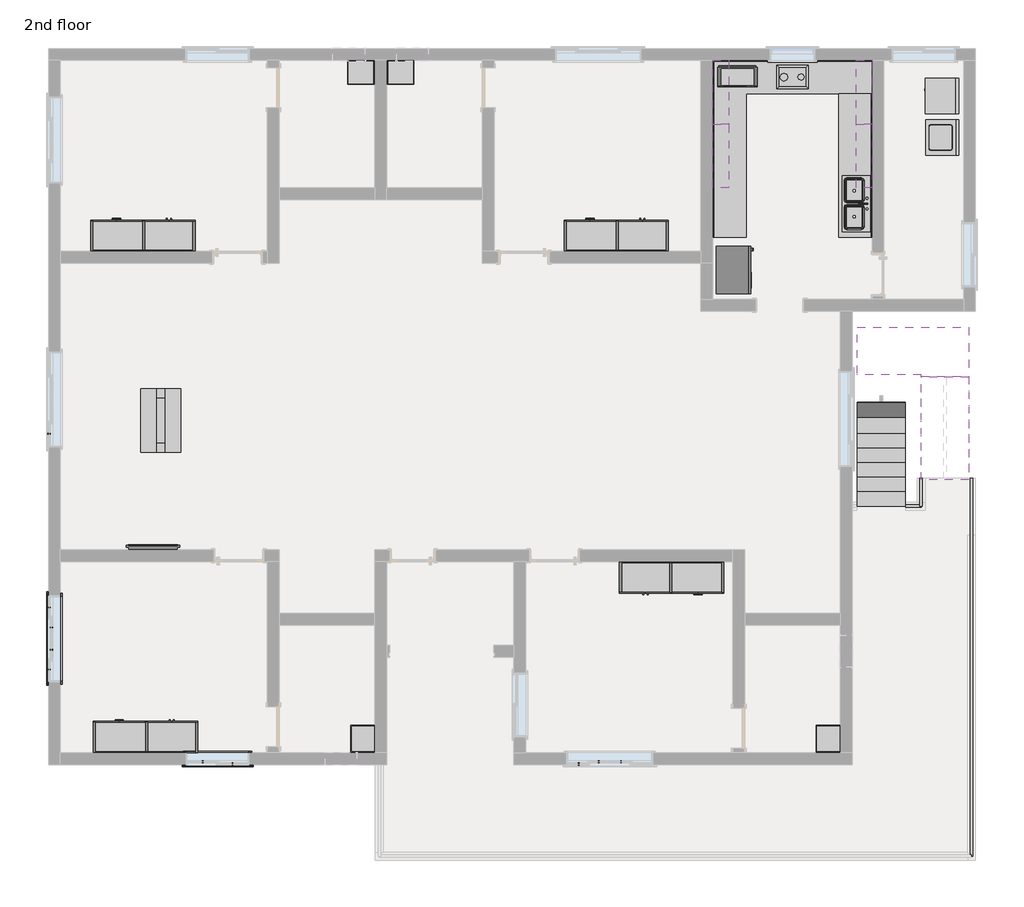
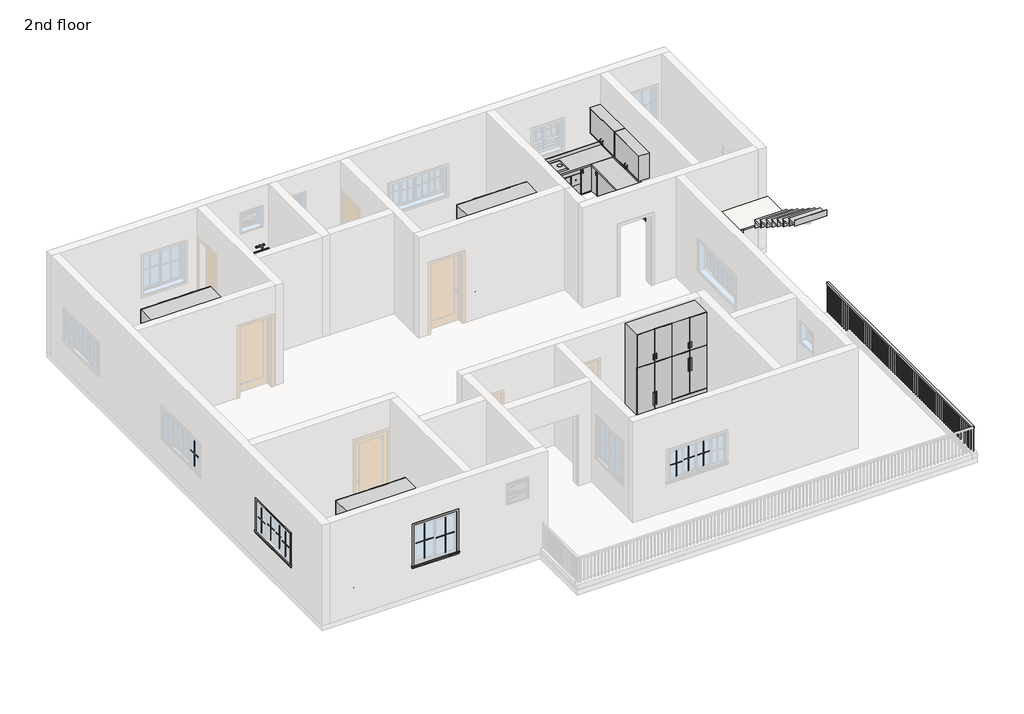
# One storey, part 3 of 4: 19 furniture elements, 18 proxies, 5 flow terminals, 3 railings, 2 stair flights, 1 slab.
"""IFC4 building model written with IfcOpenShell, lengths in millimetres."""

from ifc_helpers import new_model, si_unit, frame, origin, place, context, project, spatial, polyline, outline, extrude, transform, mapped, element, save
from components import proxy_3c1fa1d0, proxy_97c73763, proxy_e661f726, muntin_pattern_2x2_muntin_pattern_2x2_6186d23a, muntin_pattern_2x2_muntin_pattern_2x2_31a16349, muntin_pattern_2x2_muntin_pattern_2x2_cf37b409, trim_window_exterior_flat_with_sill_c3f87112, trim_window_exterior_flat_with_sill_7cfdd449, trim_window_interior_flat_picture_frame_1c33fa8a, trim_window_interior_flat_picture_frame_f1e0b15b, proxy_e75280ca, flow_terminal_cce4e9d2, flow_terminal_a53be723, furniture_65fa61b5, furniture_1wardrobe_6271_1wardrobe_6271_4dd35231, furniture_3428e43d, furniture_97fe820d, furniture_803bf5e8, furniture_2797bbf7, furniture_b6aab1a0, furniture_ea954fa4, white_modern_coffee_table_17067_white_modern_coffee_table_d4aed9ff, non_monolithic_landing_7206712e, stair_flight_52e4cb2b, stair_flight_4fb3dba1

model = new_model("IFC4")

# Units and contexts
model_context = context("Model", 3, world=origin())
ifc_project = project(units=[si_unit("LENGTHUNIT", "METRE", prefix="MILLI")], contexts=[model_context])

# Site, building, storey
site = spatial("IfcSite", under=ifc_project)
building = spatial("IfcBuilding", under=site)
storey = spatial("IfcBuildingStorey", under=building, Name="2nd floor", Elevation=7010.4)

# Proxies
placement = place(None, origin())
proxy_shape = proxy_3c1fa1d0(model_context)
element("IfcBuildingElementProxy", 1, Name="Cook Top-2 Unit : 12\" x 18\" 2", ObjectType="Cook Top-2 Unit : 12\" x 18\" 2", at=placement, inside=storey, context=model_context, shape_type="MappedRepresentation", body=[
    mapped(proxy_shape, transform((6250.0508793, 6451.6660813, 7010.4), x_axis=(0.0, 1.0, 0.0), y_axis=(-1.0, 0.0, 0.0), z_axis=(0.0, 0.0, 1.0))),
])
proxy_2_shape = proxy_97c73763(model_context)
element("IfcBuildingElementProxy", 2, Name="Dryer : 27\" x 25\" x 35\"", ObjectType="Dryer : 27\" x 25\" x 35\"", at=placement, inside=storey, context=model_context, shape_type="MappedRepresentation", body=[
    mapped(proxy_2_shape, transform((8769.6870876, 6542.578625, 7010.4), x_axis=(0.0, -1.0, 0.0), y_axis=(1.0, 0.0, 0.0), z_axis=(0.0, 0.0, 1.0))),
])
proxy_3_shape = proxy_e661f726(model_context)
element("IfcBuildingElementProxy", 3, Name="Microwave : 30\" x 16\" x 18\"", ObjectType="Microwave : 30\" x 16\" x 18\"", at=placement, inside=storey, context=model_context, shape_type="MappedRepresentation", body=[
    mapped(proxy_3_shape, transform((4665.4332064, 6893.6465872, 7010.4), x_axis=(1.0, 0.0, 0.0), y_axis=(0.0, 1.0, 0.0), z_axis=(0.0, 0.0, 1.0))),
])
muntin_pattern_2x2_muntin_pattern_2x2_shape = muntin_pattern_2x2_muntin_pattern_2x2_6186d23a(model_context)
element("IfcBuildingElementProxy", 4, Name="Muntin Pattern_2x2 : Muntin Pattern_2x2", ObjectType="Muntin Pattern_2x2 : Muntin Pattern_2x2", at=placement, inside=storey, context=model_context, shape_type="MappedRepresentation", body=[
    mapped(muntin_pattern_2x2_muntin_pattern_2x2_shape, transform((2933.7010838, -6588.0589187, 8007.35), x_axis=(-1.0, 0.0, 0.0), y_axis=(0.0, -1.0, 0.0), z_axis=(0.0, 0.0, 1.0))),
])
element("IfcBuildingElementProxy", 5, Name="Muntin Pattern_2x2 : Muntin Pattern_2x2", ObjectType="Muntin Pattern_2x2 : Muntin Pattern_2x2", at=placement, inside=storey, context=model_context, shape_type="MappedRepresentation", body=[
    mapped(muntin_pattern_2x2_muntin_pattern_2x2_shape, transform((2508.2510838, -6588.0589187, 8007.35), x_axis=(-1.0, 0.0, 0.0), y_axis=(0.0, -1.0, 0.0), z_axis=(0.0, 0.0, 1.0))),
])
element("IfcBuildingElementProxy", 6, Name="Muntin Pattern_2x2 : Muntin Pattern_2x2", ObjectType="Muntin Pattern_2x2 : Muntin Pattern_2x2", at=placement, inside=storey, context=model_context, shape_type="MappedRepresentation", body=[
    mapped(muntin_pattern_2x2_muntin_pattern_2x2_shape, transform((2127.2510838, -6632.5089187, 8007.35), x_axis=(-1.0, 0.0, 0.0), y_axis=(0.0, -1.0, 0.0), z_axis=(0.0, 0.0, 1.0))),
])
element("IfcBuildingElementProxy", 7, Name="Muntin Pattern_2x2 : Muntin Pattern_2x2", ObjectType="Muntin Pattern_2x2 : Muntin Pattern_2x2", at=placement, inside=storey, context=model_context, shape_type="MappedRepresentation", body=[
    mapped(muntin_pattern_2x2_muntin_pattern_2x2_shape, transform((-8020.0489162, -4822.7589187, 8007.35), x_axis=(0.0, 1.0, 0.0), y_axis=(-1.0, 0.0, 0.0), z_axis=(0.0, 0.0, 1.0))),
])
element("IfcBuildingElementProxy", 8, Name="Muntin Pattern_2x2 : Muntin Pattern_2x2", ObjectType="Muntin Pattern_2x2 : Muntin Pattern_2x2", at=placement, inside=storey, context=model_context, shape_type="MappedRepresentation", body=[
    mapped(muntin_pattern_2x2_muntin_pattern_2x2_shape, transform((-7975.5989162, -4441.7589187, 8007.35), x_axis=(0.0, 1.0, 0.0), y_axis=(-1.0, 0.0, 0.0), z_axis=(0.0, 0.0, 1.0))),
])
element("IfcBuildingElementProxy", 9, Name="Muntin Pattern_2x2 : Muntin Pattern_2x2", ObjectType="Muntin Pattern_2x2 : Muntin Pattern_2x2", at=placement, inside=storey, context=model_context, shape_type="MappedRepresentation", body=[
    mapped(muntin_pattern_2x2_muntin_pattern_2x2_shape, transform((-7975.5989162, -4016.3089187, 8007.35), x_axis=(0.0, 1.0, 0.0), y_axis=(-1.0, 0.0, 0.0), z_axis=(0.0, 0.0, 1.0))),
])
element("IfcBuildingElementProxy", 10, Name="Muntin Pattern_2x2 : Muntin Pattern_2x2", ObjectType="Muntin Pattern_2x2 : Muntin Pattern_2x2", at=placement, inside=storey, context=model_context, shape_type="MappedRepresentation", body=[
    mapped(muntin_pattern_2x2_muntin_pattern_2x2_shape, transform((-8020.0489162, -3635.3089187, 8007.35), x_axis=(0.0, 1.0, 0.0), y_axis=(-1.0, 0.0, 0.0), z_axis=(0.0, 0.0, 1.0))),
])
muntin_pattern_2x2_muntin_pattern_2x2_2_shape = muntin_pattern_2x2_muntin_pattern_2x2_31a16349(model_context)
element("IfcBuildingElementProxy", 11, Name="Muntin Pattern_2x2 : Muntin Pattern_2x2", ObjectType="Muntin Pattern_2x2 : Muntin Pattern_2x2", at=placement, inside=storey, context=model_context, shape_type="MappedRepresentation", body=[
    mapped(muntin_pattern_2x2_muntin_pattern_2x2_2_shape, transform((-8020.0489162, -304.7339187, 8007.35), x_axis=(0.0, 1.0, 0.0), y_axis=(-1.0, 0.0, 0.0), z_axis=(0.0, 0.0, 1.0))),
])
muntin_pattern_2x2_muntin_pattern_2x2_3_shape = muntin_pattern_2x2_muntin_pattern_2x2_cf37b409(model_context)
element("IfcBuildingElementProxy", 12, Name="Muntin Pattern_2x2 : Muntin Pattern_2x2", ObjectType="Muntin Pattern_2x2 : Muntin Pattern_2x2", at=placement, inside=storey, context=model_context, shape_type="MappedRepresentation", body=[
    mapped(muntin_pattern_2x2_muntin_pattern_2x2_3_shape, transform((-5075.2364162, -6588.0589187, 8007.35), x_axis=(-1.0, 0.0, 0.0), y_axis=(0.0, -1.0, 0.0), z_axis=(0.0, 0.0, 1.0))),
])
element("IfcBuildingElementProxy", 13, Name="Muntin Pattern_2x2 : Muntin Pattern_2x2", ObjectType="Muntin Pattern_2x2 : Muntin Pattern_2x2", at=placement, inside=storey, context=model_context, shape_type="MappedRepresentation", body=[
    mapped(muntin_pattern_2x2_muntin_pattern_2x2_3_shape, transform((-4506.9114162, -6632.5089187, 8007.35), x_axis=(-1.0, 0.0, 0.0), y_axis=(0.0, -1.0, 0.0), z_axis=(0.0, 0.0, 1.0))),
])
trim_window_exterior_flat_with_sill_shape = trim_window_exterior_flat_with_sill_c3f87112(model_context)
element("IfcBuildingElementProxy", 14, Name="Trim-Window-Exterior-Flat : with Sill", ObjectType="Trim-Window-Exterior-Flat : with Sill", at=placement, inside=storey, context=model_context, shape_type="MappedRepresentation", body=[
    mapped(trim_window_exterior_flat_with_sill_shape, transform((-8029.5739162, -4229.0339187, 8839.2), x_axis=(0.0, -1.0, 0.0), y_axis=(0.0, 0.0, 1.0), z_axis=(-1.0, 0.0, 0.0))),
])
trim_window_exterior_flat_with_sill_2_shape = trim_window_exterior_flat_with_sill_7cfdd449(model_context)
element("IfcBuildingElementProxy", 15, Name="Trim-Window-Exterior-Flat : with Sill", ObjectType="Trim-Window-Exterior-Flat : with Sill", at=placement, inside=storey, context=model_context, shape_type="MappedRepresentation", body=[
    mapped(trim_window_exterior_flat_with_sill_2_shape, transform((-4791.0739162, -6642.0339187, 9144.0), x_axis=(1.0, 0.0, 0.0), y_axis=(0.0, 0.0, 1.0), z_axis=(0.0, -1.0, 0.0))),
])
trim_window_interior_flat_picture_frame_shape = trim_window_interior_flat_picture_frame_1c33fa8a(model_context)
element("IfcBuildingElementProxy", 16, Name="Trim-Window-Interior-Flat : Picture Frame", ObjectType="Trim-Window-Interior-Flat : Picture Frame", at=placement, inside=storey, context=model_context, shape_type="MappedRepresentation", body=[
    mapped(trim_window_interior_flat_picture_frame_shape, transform((-7800.9739162, -4229.0339187, 8839.2), x_axis=(0.0, 1.0, 0.0), y_axis=(0.0, 0.0, 1.0), z_axis=(1.0, 0.0, 0.0))),
])
trim_window_interior_flat_picture_frame_2_shape = trim_window_interior_flat_picture_frame_f1e0b15b(model_context)
element("IfcBuildingElementProxy", 17, Name="Trim-Window-Interior-Flat : Picture Frame", ObjectType="Trim-Window-Interior-Flat : Picture Frame", at=placement, inside=storey, context=model_context, shape_type="MappedRepresentation", body=[
    mapped(trim_window_interior_flat_picture_frame_2_shape, transform((-4791.0739162, -6413.4339187, 9144.0), x_axis=(-1.0, 0.0, 0.0), y_axis=(0.0, 0.0, 1.0), z_axis=(0.0, 1.0, 0.0))),
])
proxy_4_shape = proxy_e75280ca(model_context)
element("IfcBuildingElementProxy", 18, Name="Washer : 27\" x 25\" x 35\"", ObjectType="Washer : 27\" x 25\" x 35\"", at=placement, inside=storey, context=model_context, shape_type="MappedRepresentation", body=[
    mapped(proxy_4_shape, transform((8810.3756486, 5789.9486128, 7010.4), x_axis=(0.0, -1.0, 0.0), y_axis=(1.0, 0.0, 0.0), z_axis=(0.0, 0.0, 1.0))),
])

# Flow terminals
flow_terminal_shape = flow_terminal_cce4e9d2(model_context)
element("IfcFlowTerminal", 19, ObjectType="Sink - Work : 20\"x18\"", at=placement, inside=storey, context=model_context, shape_type="MappedRepresentation", body=[
    mapped(flow_terminal_shape, transform((-1285.8739162, 6845.3660813, 7924.8), x_axis=(1.0, 0.0, 0.0), y_axis=(0.0, 1.0, 0.0), z_axis=(0.0, 0.0, 1.0))),
])
element("IfcFlowTerminal", 20, ObjectType="Sink - Work : 20\"x18\"", at=placement, inside=storey, context=model_context, shape_type="MappedRepresentation", body=[
    mapped(flow_terminal_shape, transform((-2047.8739162, 6845.3660813, 7924.8), x_axis=(1.0, 0.0, 0.0), y_axis=(0.0, 1.0, 0.0), z_axis=(0.0, 0.0, 1.0))),
])
element("IfcFlowTerminal", 21, ObjectType="Sink - Work : 20\"x18\"", at=placement, inside=storey, context=model_context, shape_type="MappedRepresentation", body=[
    mapped(flow_terminal_shape, transform((-1781.1739162, -6146.7339187, 7924.8), x_axis=(0.0, -1.0, 0.0), y_axis=(1.0, 0.0, 0.0), z_axis=(0.0, 0.0, 1.0))),
])
element("IfcFlowTerminal", 22, ObjectType="Sink - Work : 20\"x18\"", at=placement, inside=storey, context=model_context, shape_type="MappedRepresentation", body=[
    mapped(flow_terminal_shape, transform((7134.2260838, -6146.7339187, 7924.8), x_axis=(0.0, -1.0, 0.0), y_axis=(1.0, 0.0, 0.0), z_axis=(0.0, 0.0, 1.0))),
])
flow_terminal_2_shape = flow_terminal_a53be723(model_context)
element("IfcFlowTerminal", 23, ObjectType="Sink Kitchen-Double : 42\" x 21\"", at=placement, inside=storey, context=model_context, shape_type="MappedRepresentation", body=[
    mapped(flow_terminal_2_shape, transform((7436.6806826, 4117.8553219, 7010.4), x_axis=(0.0, -1.0, 0.0), y_axis=(1.0, 0.0, 0.0), z_axis=(0.0, 0.0, 1.0))),
])

# Furniture
furniture_shape = furniture_65fa61b5(model_context)
element("IfcFurniture", 24, at=placement, inside=storey, context=model_context, shape_type="MappedRepresentation", body=[
    mapped(furniture_shape, transform((4759.3260838, 3441.7660813, 7010.4), x_axis=(0.0, 1.0, 0.0), y_axis=(-1.0, 0.0, 0.0), z_axis=(0.0, 0.0, 1.0))),
])
furniture_1wardrobe_6271_1wardrobe_6271_shape = furniture_1wardrobe_6271_1wardrobe_6271_4dd35231(model_context)
element("IfcFurniture", 25, ObjectType="1Wardrobe_6271 : 1Wardrobe_6271", at=placement, inside=storey, context=model_context, shape_type="MappedRepresentation", body=[
    mapped(furniture_1wardrobe_6271_1wardrobe_6271_shape, transform((-5222.8739162, 3187.7660813, 7010.4), x_axis=(-1.0, 0.0, 0.0), y_axis=(0.0, -1.0, 0.0), z_axis=(0.0, 0.0, 1.0))),
])
element("IfcFurniture", 26, ObjectType="1Wardrobe_6271 : 1Wardrobe_6271", at=placement, inside=storey, context=model_context, shape_type="MappedRepresentation", body=[
    mapped(furniture_1wardrobe_6271_1wardrobe_6271_shape, transform((3844.9260838, 3187.7660813, 7010.4), x_axis=(-1.0, 0.0, 0.0), y_axis=(0.0, -1.0, 0.0), z_axis=(0.0, 0.0, 1.0))),
])
element("IfcFurniture", 27, ObjectType="1Wardrobe_6271 : 1Wardrobe_6271", at=placement, inside=storey, context=model_context, shape_type="MappedRepresentation", body=[
    mapped(furniture_1wardrobe_6271_1wardrobe_6271_shape, transform((2905.1260838, -2755.8339187, 7010.4), x_axis=(1.0, 0.0, 0.0), y_axis=(0.0, 1.0, 0.0), z_axis=(0.0, 0.0, 1.0))),
])
element("IfcFurniture", 28, ObjectType="1Wardrobe_6271 : 1Wardrobe_6271", at=placement, inside=storey, context=model_context, shape_type="MappedRepresentation", body=[
    mapped(furniture_1wardrobe_6271_1wardrobe_6271_shape, transform((-5172.0739162, -6413.4339187, 7010.4), x_axis=(-1.0, 0.0, 0.0), y_axis=(0.0, -1.0, 0.0), z_axis=(0.0, 0.0, 1.0))),
])
furniture_2_shape = furniture_3428e43d(model_context)
element("IfcFurniture", 29, ObjectType="48\" 2", at=placement, inside=storey, context=model_context, shape_type="MappedRepresentation", body=[
    mapped(furniture_2_shape, transform((6128.9811238, 6845.3660813, 7010.4), x_axis=(1.0, 0.0, 0.0), y_axis=(0.0, 1.0, 0.0), z_axis=(0.0, 0.0, 1.0))),
])
element("IfcFurniture", 30, ObjectType="48\" 2", at=placement, inside=storey, context=model_context, shape_type="MappedRepresentation", body=[
    mapped(furniture_2_shape, transform((7134.2260838, 5230.5211213, 7010.4), x_axis=(0.0, 1.0, 0.0), y_axis=(-1.0, 0.0, 0.0), z_axis=(0.0, 0.0, 1.0))),
])
element("IfcFurniture", 31, ObjectType="48\" 2", at=placement, inside=storey, context=model_context, shape_type="MappedRepresentation", body=[
    mapped(furniture_2_shape, transform((4695.8260838, 5230.5211213, 7010.4), x_axis=(0.0, 1.0, 0.0), y_axis=(-1.0, 0.0, 0.0), z_axis=(0.0, 0.0, 1.0))),
])
element("IfcFurniture", 32, ObjectType="48\" 2", at=placement, inside=storey, context=model_context, shape_type="MappedRepresentation", body=[
    mapped(furniture_2_shape, transform((4695.8260838, 4011.3211213, 7010.4), x_axis=(0.0, 1.0, 0.0), y_axis=(-1.0, 0.0, 0.0), z_axis=(0.0, 0.0, 1.0))),
])
furniture_3_shape = furniture_97fe820d(model_context)
element("IfcFurniture", 33, ObjectType="Base Cabinet-Corner Unit-Square : 36\"", at=placement, inside=storey, context=model_context, shape_type="MappedRepresentation", body=[
    mapped(furniture_3_shape, transform((7217.0883788, 6845.3660813, 7010.4), x_axis=(1.0, 0.0, 0.0), y_axis=(0.0, 1.0, 0.0), z_axis=(0.0, 0.0, 1.0))),
])
element("IfcFurniture", 34, ObjectType="Base Cabinet-Corner Unit-Square : 36\"", at=placement, inside=storey, context=model_context, shape_type="MappedRepresentation", body=[
    mapped(furniture_3_shape, transform((4695.8260838, 6318.6283764, 7010.4), x_axis=(0.0, 1.0, 0.0), y_axis=(-1.0, 0.0, 0.0), z_axis=(0.0, 0.0, 1.0))),
])
furniture_4_shape = furniture_803bf5e8(model_context)
element("IfcFurniture", 35, ObjectType="Counter Top w Sink : 24\" Depth", at=placement, inside=storey, context=model_context, shape_type="MappedRepresentation", body=[
    mapped(furniture_4_shape, transform((7743.8260838, 5009.9037862, 7010.4), x_axis=(0.0, -1.0, 0.0), y_axis=(1.0, 0.0, 0.0), z_axis=(0.0, 0.0, 1.0))),
])
furniture_5_shape = furniture_2797bbf7(model_context)
element("IfcFurniture", 36, ObjectType="Counter Top-L Shaped : 24\" Depth", at=placement, inside=storey, context=model_context, shape_type="MappedRepresentation", body=[
    mapped(furniture_5_shape, transform((5896.2883788, 6845.3660813, 7010.4), x_axis=(1.0, 0.0, 0.0), y_axis=(0.0, 1.0, 0.0), z_axis=(0.0, 0.0, 1.0))),
])
furniture_6_shape = furniture_b6aab1a0(model_context)
element("IfcFurniture", 37, ObjectType="Television-Plasma : 42\"", at=placement, inside=storey, context=model_context, shape_type="MappedRepresentation", body=[
    mapped(furniture_6_shape, transform((-5972.1739162, -2527.2339187, 8077.2), x_axis=(-1.0, 0.0, 0.0), y_axis=(0.0, -1.0, 0.0), z_axis=(0.0, 0.0, 1.0))),
])
furniture_7_shape = furniture_ea954fa4(model_context)
element("IfcFurniture", 38, ObjectType="Upper Cabinet-Pass-Thru : 48\" x 30\" x 12\"", at=placement, inside=storey, context=model_context, shape_type="MappedRepresentation", body=[
    mapped(furniture_7_shape, transform((4695.8260838, 6217.0283764, 7010.4), x_axis=(0.0, 1.0, 0.0), y_axis=(-1.0, 0.0, 0.0), z_axis=(0.0, 0.0, 1.0))),
])
element("IfcFurniture", 39, ObjectType="Upper Cabinet-Pass-Thru : 48\" x 30\" x 12\"", at=placement, inside=storey, context=model_context, shape_type="MappedRepresentation", body=[
    mapped(furniture_7_shape, transform((4695.8260838, 4997.8283764, 7010.4), x_axis=(0.0, 1.0, 0.0), y_axis=(-1.0, 0.0, 0.0), z_axis=(0.0, 0.0, 1.0))),
])
element("IfcFurniture", 40, ObjectType="Upper Cabinet-Pass-Thru : 48\" x 30\" x 12\"", at=placement, inside=storey, context=model_context, shape_type="MappedRepresentation", body=[
    mapped(furniture_7_shape, transform((7743.8260838, 6254.5037862, 7010.4), x_axis=(0.0, -1.0, 0.0), y_axis=(1.0, 0.0, 0.0), z_axis=(0.0, 0.0, 1.0))),
])
element("IfcFurniture", 41, ObjectType="Upper Cabinet-Pass-Thru : 48\" x 30\" x 12\"", at=placement, inside=storey, context=model_context, shape_type="MappedRepresentation", body=[
    mapped(furniture_7_shape, transform((7743.8260838, 5035.3037862, 7010.4), x_axis=(0.0, -1.0, 0.0), y_axis=(1.0, 0.0, 0.0), z_axis=(0.0, 0.0, 1.0))),
])
white_modern_coffee_table_17067_white_modern_coffee_table_shape = white_modern_coffee_table_17067_white_modern_coffee_table_d4aed9ff(model_context)
element("IfcFurniture", 42, ObjectType="White_Modern_Coffee_Table_17067 : White_Modern_Coffee_Table_17067", at=placement, inside=storey, context=model_context, shape_type="MappedRepresentation", body=[
    mapped(white_modern_coffee_table_17067_white_modern_coffee_table_shape, transform((-5878.4127262, -50.7339187, 7010.4), x_axis=(0.0, 1.0, 0.0), y_axis=(-1.0, 0.0, 0.0), z_axis=(0.0, 0.0, 1.0))),
])

# Railings
element("IfcRailing", 43, ObjectType="Handrail - Rectangular", at=placement, inside=storey, context=model_context, shape_type="SweptSolid", body=[
    extrude(outline(polyline([(9623.4260838, -1155.6339187), (9674.2260838, -1155.6339187), (9674.2260838, -8394.6339187), (9623.4260838, -8394.6339187), (9623.4260838, -1155.6339187)])), frame((0.0, 0.0, 7874.0), z_axis=(0.0, 0.0, 1.0), x_axis=(1.0, 0.0, 0.0)), (0.0, 0.0, 1.0), 50.8),
    extrude(outline(polyline([(9639.3010838, -8359.7089187), (9658.3510838, -8359.7089187), (9658.3510838, -8378.7589187), (9639.3010838, -8378.7589187), (9639.3010838, -8359.7089187)])), frame((0.0, 0.0, 7010.4), z_axis=(0.0, 0.0, 1.0), x_axis=(1.0, 0.0, 0.0)), (0.0, 0.0, 1.0), 863.6),
    extrude(outline(polyline([(9639.3010838, -8258.1089187), (9658.3510838, -8258.1089187), (9658.3510838, -8277.1589187), (9639.3010838, -8277.1589187), (9639.3010838, -8258.1089187)])), frame((0.0, 0.0, 7010.4), z_axis=(0.0, 0.0, 1.0), x_axis=(1.0, 0.0, 0.0)), (0.0, 0.0, 1.0), 863.6),
    extrude(outline(polyline([(9639.3010838, -8156.5089187), (9658.3510838, -8156.5089187), (9658.3510838, -8175.5589187), (9639.3010838, -8175.5589187), (9639.3010838, -8156.5089187)])), frame((0.0, 0.0, 7010.4), z_axis=(0.0, 0.0, 1.0), x_axis=(1.0, 0.0, 0.0)), (0.0, 0.0, 1.0), 863.6),
    extrude(outline(polyline([(9639.3010838, -8054.9089187), (9658.3510838, -8054.9089187), (9658.3510838, -8073.9589187), (9639.3010838, -8073.9589187), (9639.3010838, -8054.9089187)])), frame((0.0, 0.0, 7010.4), z_axis=(0.0, 0.0, 1.0), x_axis=(1.0, 0.0, 0.0)), (0.0, 0.0, 1.0), 863.6),
    extrude(outline(polyline([(9639.3010838, -7953.3089187), (9658.3510838, -7953.3089187), (9658.3510838, -7972.3589187), (9639.3010838, -7972.3589187), (9639.3010838, -7953.3089187)])), frame((0.0, 0.0, 7010.4), z_axis=(0.0, 0.0, 1.0), x_axis=(1.0, 0.0, 0.0)), (0.0, 0.0, 1.0), 863.6),
    extrude(outline(polyline([(9639.3010838, -7851.7089187), (9658.3510838, -7851.7089187), (9658.3510838, -7870.7589187), (9639.3010838, -7870.7589187), (9639.3010838, -7851.7089187)])), frame((0.0, 0.0, 7010.4), z_axis=(0.0, 0.0, 1.0), x_axis=(1.0, 0.0, 0.0)), (0.0, 0.0, 1.0), 863.6),
    extrude(outline(polyline([(9639.3010838, -7750.1089187), (9658.3510838, -7750.1089187), (9658.3510838, -7769.1589187), (9639.3010838, -7769.1589187), (9639.3010838, -7750.1089187)])), frame((0.0, 0.0, 7010.4), z_axis=(0.0, 0.0, 1.0), x_axis=(1.0, 0.0, 0.0)), (0.0, 0.0, 1.0), 863.6),
    extrude(outline(polyline([(9639.3010838, -7648.5089187), (9658.3510838, -7648.5089187), (9658.3510838, -7667.5589187), (9639.3010838, -7667.5589187), (9639.3010838, -7648.5089187)])), frame((0.0, 0.0, 7010.4), z_axis=(0.0, 0.0, 1.0), x_axis=(1.0, 0.0, 0.0)), (0.0, 0.0, 1.0), 863.6),
    extrude(outline(polyline([(9639.3010838, -7546.9089187), (9658.3510838, -7546.9089187), (9658.3510838, -7565.9589187), (9639.3010838, -7565.9589187), (9639.3010838, -7546.9089187)])), frame((0.0, 0.0, 7010.4), z_axis=(0.0, 0.0, 1.0), x_axis=(1.0, 0.0, 0.0)), (0.0, 0.0, 1.0), 863.6),
    extrude(outline(polyline([(9639.3010838, -7445.3089187), (9658.3510838, -7445.3089187), (9658.3510838, -7464.3589187), (9639.3010838, -7464.3589187), (9639.3010838, -7445.3089187)])), frame((0.0, 0.0, 7010.4), z_axis=(0.0, 0.0, 1.0), x_axis=(1.0, 0.0, 0.0)), (0.0, 0.0, 1.0), 863.6),
    extrude(outline(polyline([(9639.3010838, -7343.7089187), (9658.3510838, -7343.7089187), (9658.3510838, -7362.7589187), (9639.3010838, -7362.7589187), (9639.3010838, -7343.7089187)])), frame((0.0, 0.0, 7010.4), z_axis=(0.0, 0.0, 1.0), x_axis=(1.0, 0.0, 0.0)), (0.0, 0.0, 1.0), 863.6),
    extrude(outline(polyline([(9639.3010838, -7242.1089187), (9658.3510838, -7242.1089187), (9658.3510838, -7261.1589187), (9639.3010838, -7261.1589187), (9639.3010838, -7242.1089187)])), frame((0.0, 0.0, 7010.4), z_axis=(0.0, 0.0, 1.0), x_axis=(1.0, 0.0, 0.0)), (0.0, 0.0, 1.0), 863.6),
    extrude(outline(polyline([(9639.3010838, -7140.5089187), (9658.3510838, -7140.5089187), (9658.3510838, -7159.5589187), (9639.3010838, -7159.5589187), (9639.3010838, -7140.5089187)])), frame((0.0, 0.0, 7010.4), z_axis=(0.0, 0.0, 1.0), x_axis=(1.0, 0.0, 0.0)), (0.0, 0.0, 1.0), 863.6),
    extrude(outline(polyline([(9639.3010838, -7038.9089187), (9658.3510838, -7038.9089187), (9658.3510838, -7057.9589187), (9639.3010838, -7057.9589187), (9639.3010838, -7038.9089187)])), frame((0.0, 0.0, 7010.4), z_axis=(0.0, 0.0, 1.0), x_axis=(1.0, 0.0, 0.0)), (0.0, 0.0, 1.0), 863.6),
    extrude(outline(polyline([(9639.3010838, -6937.3089187), (9658.3510838, -6937.3089187), (9658.3510838, -6956.3589187), (9639.3010838, -6956.3589187), (9639.3010838, -6937.3089187)])), frame((0.0, 0.0, 7010.4), z_axis=(0.0, 0.0, 1.0), x_axis=(1.0, 0.0, 0.0)), (0.0, 0.0, 1.0), 863.6),
    extrude(outline(polyline([(9639.3010838, -6835.7089187), (9658.3510838, -6835.7089187), (9658.3510838, -6854.7589187), (9639.3010838, -6854.7589187), (9639.3010838, -6835.7089187)])), frame((0.0, 0.0, 7010.4), z_axis=(0.0, 0.0, 1.0), x_axis=(1.0, 0.0, 0.0)), (0.0, 0.0, 1.0), 863.6),
    extrude(outline(polyline([(9639.3010838, -6734.1089187), (9658.3510838, -6734.1089187), (9658.3510838, -6753.1589187), (9639.3010838, -6753.1589187), (9639.3010838, -6734.1089187)])), frame((0.0, 0.0, 7010.4), z_axis=(0.0, 0.0, 1.0), x_axis=(1.0, 0.0, 0.0)), (0.0, 0.0, 1.0), 863.6),
    extrude(outline(polyline([(9639.3010838, -6632.5089187), (9658.3510838, -6632.5089187), (9658.3510838, -6651.5589187), (9639.3010838, -6651.5589187), (9639.3010838, -6632.5089187)])), frame((0.0, 0.0, 7010.4), z_axis=(0.0, 0.0, 1.0), x_axis=(1.0, 0.0, 0.0)), (0.0, 0.0, 1.0), 863.6),
    extrude(outline(polyline([(9639.3010838, -6530.9089187), (9658.3510838, -6530.9089187), (9658.3510838, -6549.9589187), (9639.3010838, -6549.9589187), (9639.3010838, -6530.9089187)])), frame((0.0, 0.0, 7010.4), z_axis=(0.0, 0.0, 1.0), x_axis=(1.0, 0.0, 0.0)), (0.0, 0.0, 1.0), 863.6),
    extrude(outline(polyline([(9639.3010838, -6429.3089187), (9658.3510838, -6429.3089187), (9658.3510838, -6448.3589187), (9639.3010838, -6448.3589187), (9639.3010838, -6429.3089187)])), frame((0.0, 0.0, 7010.4), z_axis=(0.0, 0.0, 1.0), x_axis=(1.0, 0.0, 0.0)), (0.0, 0.0, 1.0), 863.6),
    extrude(outline(polyline([(9639.3010838, -6327.7089187), (9658.3510838, -6327.7089187), (9658.3510838, -6346.7589187), (9639.3010838, -6346.7589187), (9639.3010838, -6327.7089187)])), frame((0.0, 0.0, 7010.4), z_axis=(0.0, 0.0, 1.0), x_axis=(1.0, 0.0, 0.0)), (0.0, 0.0, 1.0), 863.6),
    extrude(outline(polyline([(9639.3010838, -6226.1089187), (9658.3510838, -6226.1089187), (9658.3510838, -6245.1589187), (9639.3010838, -6245.1589187), (9639.3010838, -6226.1089187)])), frame((0.0, 0.0, 7010.4), z_axis=(0.0, 0.0, 1.0), x_axis=(1.0, 0.0, 0.0)), (0.0, 0.0, 1.0), 863.6),
    extrude(outline(polyline([(9639.3010838, -6124.5089187), (9658.3510838, -6124.5089187), (9658.3510838, -6143.5589187), (9639.3010838, -6143.5589187), (9639.3010838, -6124.5089187)])), frame((0.0, 0.0, 7010.4), z_axis=(0.0, 0.0, 1.0), x_axis=(1.0, 0.0, 0.0)), (0.0, 0.0, 1.0), 863.6),
    extrude(outline(polyline([(9639.3010838, -6022.9089187), (9658.3510838, -6022.9089187), (9658.3510838, -6041.9589187), (9639.3010838, -6041.9589187), (9639.3010838, -6022.9089187)])), frame((0.0, 0.0, 7010.4), z_axis=(0.0, 0.0, 1.0), x_axis=(1.0, 0.0, 0.0)), (0.0, 0.0, 1.0), 863.6),
    extrude(outline(polyline([(9639.3010838, -5921.3089187), (9658.3510838, -5921.3089187), (9658.3510838, -5940.3589187), (9639.3010838, -5940.3589187), (9639.3010838, -5921.3089187)])), frame((0.0, 0.0, 7010.4), z_axis=(0.0, 0.0, 1.0), x_axis=(1.0, 0.0, 0.0)), (0.0, 0.0, 1.0), 863.6),
    extrude(outline(polyline([(9639.3010838, -5819.7089187), (9658.3510838, -5819.7089187), (9658.3510838, -5838.7589187), (9639.3010838, -5838.7589187), (9639.3010838, -5819.7089187)])), frame((0.0, 0.0, 7010.4), z_axis=(0.0, 0.0, 1.0), x_axis=(1.0, 0.0, 0.0)), (0.0, 0.0, 1.0), 863.6),
    extrude(outline(polyline([(9639.3010838, -5718.1089187), (9658.3510838, -5718.1089187), (9658.3510838, -5737.1589187), (9639.3010838, -5737.1589187), (9639.3010838, -5718.1089187)])), frame((0.0, 0.0, 7010.4), z_axis=(0.0, 0.0, 1.0), x_axis=(1.0, 0.0, 0.0)), (0.0, 0.0, 1.0), 863.6),
    extrude(outline(polyline([(9639.3010838, -5616.5089187), (9658.3510838, -5616.5089187), (9658.3510838, -5635.5589187), (9639.3010838, -5635.5589187), (9639.3010838, -5616.5089187)])), frame((0.0, 0.0, 7010.4), z_axis=(0.0, 0.0, 1.0), x_axis=(1.0, 0.0, 0.0)), (0.0, 0.0, 1.0), 863.6),
    extrude(outline(polyline([(9639.3010838, -5514.9089187), (9658.3510838, -5514.9089187), (9658.3510838, -5533.9589187), (9639.3010838, -5533.9589187), (9639.3010838, -5514.9089187)])), frame((0.0, 0.0, 7010.4), z_axis=(0.0, 0.0, 1.0), x_axis=(1.0, 0.0, 0.0)), (0.0, 0.0, 1.0), 863.6),
    extrude(outline(polyline([(9639.3010838, -5413.3089187), (9658.3510838, -5413.3089187), (9658.3510838, -5432.3589187), (9639.3010838, -5432.3589187), (9639.3010838, -5413.3089187)])), frame((0.0, 0.0, 7010.4), z_axis=(0.0, 0.0, 1.0), x_axis=(1.0, 0.0, 0.0)), (0.0, 0.0, 1.0), 863.6),
    extrude(outline(polyline([(9639.3010838, -5311.7089187), (9658.3510838, -5311.7089187), (9658.3510838, -5330.7589187), (9639.3010838, -5330.7589187), (9639.3010838, -5311.7089187)])), frame((0.0, 0.0, 7010.4), z_axis=(0.0, 0.0, 1.0), x_axis=(1.0, 0.0, 0.0)), (0.0, 0.0, 1.0), 863.6),
    extrude(outline(polyline([(9639.3010838, -5210.1089187), (9658.3510838, -5210.1089187), (9658.3510838, -5229.1589187), (9639.3010838, -5229.1589187), (9639.3010838, -5210.1089187)])), frame((0.0, 0.0, 7010.4), z_axis=(0.0, 0.0, 1.0), x_axis=(1.0, 0.0, 0.0)), (0.0, 0.0, 1.0), 863.6),
    extrude(outline(polyline([(9639.3010838, -5108.5089187), (9658.3510838, -5108.5089187), (9658.3510838, -5127.5589187), (9639.3010838, -5127.5589187), (9639.3010838, -5108.5089187)])), frame((0.0, 0.0, 7010.4), z_axis=(0.0, 0.0, 1.0), x_axis=(1.0, 0.0, 0.0)), (0.0, 0.0, 1.0), 863.6),
    extrude(outline(polyline([(9639.3010838, -5006.9089187), (9658.3510838, -5006.9089187), (9658.3510838, -5025.9589187), (9639.3010838, -5025.9589187), (9639.3010838, -5006.9089187)])), frame((0.0, 0.0, 7010.4), z_axis=(0.0, 0.0, 1.0), x_axis=(1.0, 0.0, 0.0)), (0.0, 0.0, 1.0), 863.6),
    extrude(outline(polyline([(9639.3010838, -4905.3089187), (9658.3510838, -4905.3089187), (9658.3510838, -4924.3589187), (9639.3010838, -4924.3589187), (9639.3010838, -4905.3089187)])), frame((0.0, 0.0, 7010.4), z_axis=(0.0, 0.0, 1.0), x_axis=(1.0, 0.0, 0.0)), (0.0, 0.0, 1.0), 863.6),
    extrude(outline(polyline([(9639.3010838, -4803.7089187), (9658.3510838, -4803.7089187), (9658.3510838, -4822.7589187), (9639.3010838, -4822.7589187), (9639.3010838, -4803.7089187)])), frame((0.0, 0.0, 7010.4), z_axis=(0.0, 0.0, 1.0), x_axis=(1.0, 0.0, 0.0)), (0.0, 0.0, 1.0), 863.6),
    extrude(outline(polyline([(9639.3010838, -4702.1089187), (9658.3510838, -4702.1089187), (9658.3510838, -4721.1589187), (9639.3010838, -4721.1589187), (9639.3010838, -4702.1089187)])), frame((0.0, 0.0, 7010.4), z_axis=(0.0, 0.0, 1.0), x_axis=(1.0, 0.0, 0.0)), (0.0, 0.0, 1.0), 863.6),
    extrude(outline(polyline([(9639.3010838, -4600.5089187), (9658.3510838, -4600.5089187), (9658.3510838, -4619.5589187), (9639.3010838, -4619.5589187), (9639.3010838, -4600.5089187)])), frame((0.0, 0.0, 7010.4), z_axis=(0.0, 0.0, 1.0), x_axis=(1.0, 0.0, 0.0)), (0.0, 0.0, 1.0), 863.6),
    extrude(outline(polyline([(9639.3010838, -4498.9089187), (9658.3510838, -4498.9089187), (9658.3510838, -4517.9589187), (9639.3010838, -4517.9589187), (9639.3010838, -4498.9089187)])), frame((0.0, 0.0, 7010.4), z_axis=(0.0, 0.0, 1.0), x_axis=(1.0, 0.0, 0.0)), (0.0, 0.0, 1.0), 863.6),
    extrude(outline(polyline([(9639.3010838, -4397.3089187), (9658.3510838, -4397.3089187), (9658.3510838, -4416.3589187), (9639.3010838, -4416.3589187), (9639.3010838, -4397.3089187)])), frame((0.0, 0.0, 7010.4), z_axis=(0.0, 0.0, 1.0), x_axis=(1.0, 0.0, 0.0)), (0.0, 0.0, 1.0), 863.6),
    extrude(outline(polyline([(9639.3010838, -4295.7089187), (9658.3510838, -4295.7089187), (9658.3510838, -4314.7589187), (9639.3010838, -4314.7589187), (9639.3010838, -4295.7089187)])), frame((0.0, 0.0, 7010.4), z_axis=(0.0, 0.0, 1.0), x_axis=(1.0, 0.0, 0.0)), (0.0, 0.0, 1.0), 863.6),
    extrude(outline(polyline([(9639.3010838, -4194.1089187), (9658.3510838, -4194.1089187), (9658.3510838, -4213.1589187), (9639.3010838, -4213.1589187), (9639.3010838, -4194.1089187)])), frame((0.0, 0.0, 7010.4), z_axis=(0.0, 0.0, 1.0), x_axis=(1.0, 0.0, 0.0)), (0.0, 0.0, 1.0), 863.6),
    extrude(outline(polyline([(9639.3010838, -4092.5089187), (9658.3510838, -4092.5089187), (9658.3510838, -4111.5589187), (9639.3010838, -4111.5589187), (9639.3010838, -4092.5089187)])), frame((0.0, 0.0, 7010.4), z_axis=(0.0, 0.0, 1.0), x_axis=(1.0, 0.0, 0.0)), (0.0, 0.0, 1.0), 863.6),
    extrude(outline(polyline([(9639.3010838, -3990.9089187), (9658.3510838, -3990.9089187), (9658.3510838, -4009.9589187), (9639.3010838, -4009.9589187), (9639.3010838, -3990.9089187)])), frame((0.0, 0.0, 7010.4), z_axis=(0.0, 0.0, 1.0), x_axis=(1.0, 0.0, 0.0)), (0.0, 0.0, 1.0), 863.6),
    extrude(outline(polyline([(9639.3010838, -3889.3089187), (9658.3510838, -3889.3089187), (9658.3510838, -3908.3589187), (9639.3010838, -3908.3589187), (9639.3010838, -3889.3089187)])), frame((0.0, 0.0, 7010.4), z_axis=(0.0, 0.0, 1.0), x_axis=(1.0, 0.0, 0.0)), (0.0, 0.0, 1.0), 863.6),
    extrude(outline(polyline([(9639.3010838, -3787.7089187), (9658.3510838, -3787.7089187), (9658.3510838, -3806.7589187), (9639.3010838, -3806.7589187), (9639.3010838, -3787.7089187)])), frame((0.0, 0.0, 7010.4), z_axis=(0.0, 0.0, 1.0), x_axis=(1.0, 0.0, 0.0)), (0.0, 0.0, 1.0), 863.6),
    extrude(outline(polyline([(9639.3010838, -3686.1089187), (9658.3510838, -3686.1089187), (9658.3510838, -3705.1589187), (9639.3010838, -3705.1589187), (9639.3010838, -3686.1089187)])), frame((0.0, 0.0, 7010.4), z_axis=(0.0, 0.0, 1.0), x_axis=(1.0, 0.0, 0.0)), (0.0, 0.0, 1.0), 863.6),
    extrude(outline(polyline([(9639.3010838, -3584.5089187), (9658.3510838, -3584.5089187), (9658.3510838, -3603.5589187), (9639.3010838, -3603.5589187), (9639.3010838, -3584.5089187)])), frame((0.0, 0.0, 7010.4), z_axis=(0.0, 0.0, 1.0), x_axis=(1.0, 0.0, 0.0)), (0.0, 0.0, 1.0), 863.6),
    extrude(outline(polyline([(9639.3010838, -3482.9089187), (9658.3510838, -3482.9089187), (9658.3510838, -3501.9589187), (9639.3010838, -3501.9589187), (9639.3010838, -3482.9089187)])), frame((0.0, 0.0, 7010.4), z_axis=(0.0, 0.0, 1.0), x_axis=(1.0, 0.0, 0.0)), (0.0, 0.0, 1.0), 863.6),
    extrude(outline(polyline([(9639.3010838, -3381.3089187), (9658.3510838, -3381.3089187), (9658.3510838, -3400.3589187), (9639.3010838, -3400.3589187), (9639.3010838, -3381.3089187)])), frame((0.0, 0.0, 7010.4), z_axis=(0.0, 0.0, 1.0), x_axis=(1.0, 0.0, 0.0)), (0.0, 0.0, 1.0), 863.6),
    extrude(outline(polyline([(9639.3010838, -3279.7089187), (9658.3510838, -3279.7089187), (9658.3510838, -3298.7589187), (9639.3010838, -3298.7589187), (9639.3010838, -3279.7089187)])), frame((0.0, 0.0, 7010.4), z_axis=(0.0, 0.0, 1.0), x_axis=(1.0, 0.0, 0.0)), (0.0, 0.0, 1.0), 863.6),
    extrude(outline(polyline([(9639.3010838, -3178.1089187), (9658.3510838, -3178.1089187), (9658.3510838, -3197.1589187), (9639.3010838, -3197.1589187), (9639.3010838, -3178.1089187)])), frame((0.0, 0.0, 7010.4), z_axis=(0.0, 0.0, 1.0), x_axis=(1.0, 0.0, 0.0)), (0.0, 0.0, 1.0), 863.6),
    extrude(outline(polyline([(9639.3010838, -3076.5089187), (9658.3510838, -3076.5089187), (9658.3510838, -3095.5589187), (9639.3010838, -3095.5589187), (9639.3010838, -3076.5089187)])), frame((0.0, 0.0, 7010.4), z_axis=(0.0, 0.0, 1.0), x_axis=(1.0, 0.0, 0.0)), (0.0, 0.0, 1.0), 863.6),
    extrude(outline(polyline([(9639.3010838, -2974.9089187), (9658.3510838, -2974.9089187), (9658.3510838, -2993.9589187), (9639.3010838, -2993.9589187), (9639.3010838, -2974.9089187)])), frame((0.0, 0.0, 7010.4), z_axis=(0.0, 0.0, 1.0), x_axis=(1.0, 0.0, 0.0)), (0.0, 0.0, 1.0), 863.6),
    extrude(outline(polyline([(9639.3010838, -2873.3089187), (9658.3510838, -2873.3089187), (9658.3510838, -2892.3589187), (9639.3010838, -2892.3589187), (9639.3010838, -2873.3089187)])), frame((0.0, 0.0, 7010.4), z_axis=(0.0, 0.0, 1.0), x_axis=(1.0, 0.0, 0.0)), (0.0, 0.0, 1.0), 863.6),
    extrude(outline(polyline([(9639.3010838, -2771.7089187), (9658.3510838, -2771.7089187), (9658.3510838, -2790.7589187), (9639.3010838, -2790.7589187), (9639.3010838, -2771.7089187)])), frame((0.0, 0.0, 7010.4), z_axis=(0.0, 0.0, 1.0), x_axis=(1.0, 0.0, 0.0)), (0.0, 0.0, 1.0), 863.6),
    extrude(outline(polyline([(9639.3010838, -2670.1089187), (9658.3510838, -2670.1089187), (9658.3510838, -2689.1589187), (9639.3010838, -2689.1589187), (9639.3010838, -2670.1089187)])), frame((0.0, 0.0, 7010.4), z_axis=(0.0, 0.0, 1.0), x_axis=(1.0, 0.0, 0.0)), (0.0, 0.0, 1.0), 863.6),
    extrude(outline(polyline([(9639.3010838, -2568.5089187), (9658.3510838, -2568.5089187), (9658.3510838, -2587.5589187), (9639.3010838, -2587.5589187), (9639.3010838, -2568.5089187)])), frame((0.0, 0.0, 7010.4), z_axis=(0.0, 0.0, 1.0), x_axis=(1.0, 0.0, 0.0)), (0.0, 0.0, 1.0), 863.6),
    extrude(outline(polyline([(9639.3010838, -2466.9089187), (9658.3510838, -2466.9089187), (9658.3510838, -2485.9589187), (9639.3010838, -2485.9589187), (9639.3010838, -2466.9089187)])), frame((0.0, 0.0, 7010.4), z_axis=(0.0, 0.0, 1.0), x_axis=(1.0, 0.0, 0.0)), (0.0, 0.0, 1.0), 863.6),
    extrude(outline(polyline([(9639.3010838, -2365.3089187), (9658.3510838, -2365.3089187), (9658.3510838, -2384.3589187), (9639.3010838, -2384.3589187), (9639.3010838, -2365.3089187)])), frame((0.0, 0.0, 7010.4), z_axis=(0.0, 0.0, 1.0), x_axis=(1.0, 0.0, 0.0)), (0.0, 0.0, 1.0), 863.6),
    extrude(outline(polyline([(9639.3010838, -2263.7089187), (9658.3510838, -2263.7089187), (9658.3510838, -2282.7589187), (9639.3010838, -2282.7589187), (9639.3010838, -2263.7089187)])), frame((0.0, 0.0, 7010.4), z_axis=(0.0, 0.0, 1.0), x_axis=(1.0, 0.0, 0.0)), (0.0, 0.0, 1.0), 863.6),
    extrude(outline(polyline([(9639.3010838, -2162.1089187), (9658.3510838, -2162.1089187), (9658.3510838, -2181.1589187), (9639.3010838, -2181.1589187), (9639.3010838, -2162.1089187)])), frame((0.0, 0.0, 7010.4), z_axis=(0.0, 0.0, 1.0), x_axis=(1.0, 0.0, 0.0)), (0.0, 0.0, 1.0), 863.6),
    extrude(outline(polyline([(9639.3010838, -2060.5089187), (9658.3510838, -2060.5089187), (9658.3510838, -2079.5589187), (9639.3010838, -2079.5589187), (9639.3010838, -2060.5089187)])), frame((0.0, 0.0, 7010.4), z_axis=(0.0, 0.0, 1.0), x_axis=(1.0, 0.0, 0.0)), (0.0, 0.0, 1.0), 863.6),
    extrude(outline(polyline([(9639.3010838, -1958.9089187), (9658.3510838, -1958.9089187), (9658.3510838, -1977.9589187), (9639.3010838, -1977.9589187), (9639.3010838, -1958.9089187)])), frame((0.0, 0.0, 7010.4), z_axis=(0.0, 0.0, 1.0), x_axis=(1.0, 0.0, 0.0)), (0.0, 0.0, 1.0), 863.6),
    extrude(outline(polyline([(9639.3010838, -1857.3089187), (9658.3510838, -1857.3089187), (9658.3510838, -1876.3589187), (9639.3010838, -1876.3589187), (9639.3010838, -1857.3089187)])), frame((0.0, 0.0, 7010.4), z_axis=(0.0, 0.0, 1.0), x_axis=(1.0, 0.0, 0.0)), (0.0, 0.0, 1.0), 863.6),
    extrude(outline(polyline([(9639.3010838, -1755.7089187), (9658.3510838, -1755.7089187), (9658.3510838, -1774.7589187), (9639.3010838, -1774.7589187), (9639.3010838, -1755.7089187)])), frame((0.0, 0.0, 7010.4), z_axis=(0.0, 0.0, 1.0), x_axis=(1.0, 0.0, 0.0)), (0.0, 0.0, 1.0), 863.6),
    extrude(outline(polyline([(9639.3010838, -1654.1089187), (9658.3510838, -1654.1089187), (9658.3510838, -1673.1589187), (9639.3010838, -1673.1589187), (9639.3010838, -1654.1089187)])), frame((0.0, 0.0, 7010.4), z_axis=(0.0, 0.0, 1.0), x_axis=(1.0, 0.0, 0.0)), (0.0, 0.0, 1.0), 863.6),
    extrude(outline(polyline([(9639.3010838, -1552.5089187), (9658.3510838, -1552.5089187), (9658.3510838, -1571.5589187), (9639.3010838, -1571.5589187), (9639.3010838, -1552.5089187)])), frame((0.0, 0.0, 7010.4), z_axis=(0.0, 0.0, 1.0), x_axis=(1.0, 0.0, 0.0)), (0.0, 0.0, 1.0), 863.6),
    extrude(outline(polyline([(9639.3010838, -1450.9089187), (9658.3510838, -1450.9089187), (9658.3510838, -1469.9589187), (9639.3010838, -1469.9589187), (9639.3010838, -1450.9089187)])), frame((0.0, 0.0, 7010.4), z_axis=(0.0, 0.0, 1.0), x_axis=(1.0, 0.0, 0.0)), (0.0, 0.0, 1.0), 863.6),
    extrude(outline(polyline([(9639.3010838, -1349.3089187), (9658.3510838, -1349.3089187), (9658.3510838, -1368.3589187), (9639.3010838, -1368.3589187), (9639.3010838, -1349.3089187)])), frame((0.0, 0.0, 7010.4), z_axis=(0.0, 0.0, 1.0), x_axis=(1.0, 0.0, 0.0)), (0.0, 0.0, 1.0), 863.6),
    extrude(outline(polyline([(9639.3010838, -1247.7089187), (9658.3510838, -1247.7089187), (9658.3510838, -1266.7589187), (9639.3010838, -1266.7589187), (9639.3010838, -1247.7089187)])), frame((0.0, 0.0, 7010.4), z_axis=(0.0, 0.0, 1.0), x_axis=(1.0, 0.0, 0.0)), (0.0, 0.0, 1.0), 863.6),
    extrude(outline(polyline([(9639.3010838, -8375.5839187), (9658.3510838, -8375.5839187), (9658.3510838, -8394.6339187), (9639.3010838, -8394.6339187), (9639.3010838, -8375.5839187)])), frame((0.0, 0.0, 7010.4), z_axis=(0.0, 0.0, 1.0), x_axis=(1.0, 0.0, 0.0)), (0.0, 0.0, 1.0), 863.6),
    extrude(outline(polyline([(9639.3010838, -1155.6339187), (9658.3510838, -1155.6339187), (9658.3510838, -1174.6839187), (9639.3010838, -1174.6839187), (9639.3010838, -1155.6339187)])), frame((0.0, 0.0, 7010.4), z_axis=(0.0, 0.0, 1.0), x_axis=(1.0, 0.0, 0.0)), (0.0, 0.0, 1.0), 863.6),
])
element("IfcRailing", 44, ObjectType="Handrail - Rectangular", at=placement, inside=storey, context=model_context, shape_type="SweptSolid", body=[
    extrude(outline(polyline([(8658.2260838, -1156.9972984), (8709.0260838, -1156.9972984), (8709.0260838, -1689.0339187), (8658.2260838, -1689.0339187), (8658.2260838, -1156.9972984)])), frame((0.0, 0.0, 7874.0), z_axis=(0.0, 0.0, 1.0), x_axis=(1.0, 0.0, 0.0)), (0.0, 0.0, 1.0), 50.8),
    extrude(outline(polyline([(8674.1010838, -1655.4722984), (8693.1510838, -1655.4722984), (8693.1510838, -1674.5222984), (8674.1010838, -1674.5222984), (8674.1010838, -1655.4722984)])), frame((0.0, 0.0, 7010.4), z_axis=(0.0, 0.0, 1.0), x_axis=(1.0, 0.0, 0.0)), (0.0, 0.0, 1.0), 863.6),
    extrude(outline(polyline([(8674.1010838, -1553.8722984), (8693.1510838, -1553.8722984), (8693.1510838, -1572.9222984), (8674.1010838, -1572.9222984), (8674.1010838, -1553.8722984)])), frame((0.0, 0.0, 7010.4), z_axis=(0.0, 0.0, 1.0), x_axis=(1.0, 0.0, 0.0)), (0.0, 0.0, 1.0), 863.6),
    extrude(outline(polyline([(8674.1010838, -1452.2722984), (8693.1510838, -1452.2722984), (8693.1510838, -1471.3222984), (8674.1010838, -1471.3222984), (8674.1010838, -1452.2722984)])), frame((0.0, 0.0, 7010.4), z_axis=(0.0, 0.0, 1.0), x_axis=(1.0, 0.0, 0.0)), (0.0, 0.0, 1.0), 863.6),
    extrude(outline(polyline([(8674.1010838, -1350.6722984), (8693.1510838, -1350.6722984), (8693.1510838, -1369.7222984), (8674.1010838, -1369.7222984), (8674.1010838, -1350.6722984)])), frame((0.0, 0.0, 7010.4), z_axis=(0.0, 0.0, 1.0), x_axis=(1.0, 0.0, 0.0)), (0.0, 0.0, 1.0), 863.6),
    extrude(outline(polyline([(8674.1010838, -1249.0722984), (8693.1510838, -1249.0722984), (8693.1510838, -1268.1222984), (8674.1010838, -1268.1222984), (8674.1010838, -1249.0722984)])), frame((0.0, 0.0, 7010.4), z_axis=(0.0, 0.0, 1.0), x_axis=(1.0, 0.0, 0.0)), (0.0, 0.0, 1.0), 863.6),
    extrude(outline(polyline([(8674.1010838, -1669.9839187), (8693.1510838, -1669.9839187), (8693.1510838, -1689.0339187), (8674.1010838, -1689.0339187), (8674.1010838, -1669.9839187)])), frame((0.0, 0.0, 7010.4), z_axis=(0.0, 0.0, 1.0), x_axis=(1.0, 0.0, 0.0)), (0.0, 0.0, 1.0), 863.6),
    extrude(outline(polyline([(8674.1010838, -1156.9972984), (8693.1510838, -1156.9972984), (8693.1510838, -1176.0472984), (8674.1010838, -1176.0472984), (8674.1010838, -1156.9972984)])), frame((0.0, 0.0, 7010.4), z_axis=(0.0, 0.0, 1.0), x_axis=(1.0, 0.0, 0.0)), (0.0, 0.0, 1.0), 863.6),
])
element("IfcRailing", 45, ObjectType="Handrail - Rectangular", at=placement, inside=storey, context=model_context, shape_type="SweptSolid", body=[
    extrude(outline(polyline([(8683.6260838, -1663.6339187), (8683.6260838, -1714.4339187), (8391.5260838, -1714.4339187), (8391.5260838, -1663.6339187), (8683.6260838, -1663.6339187)])), frame((0.0, 0.0, 7874.0), z_axis=(0.0, 0.0, 1.0), x_axis=(1.0, 0.0, 0.0)), (0.0, 0.0, 1.0), 50.8),
    extrude(outline(polyline([(8489.9510838, -1679.5089187), (8489.9510838, -1698.5589187), (8470.9010838, -1698.5589187), (8470.9010838, -1679.5089187), (8489.9510838, -1679.5089187)])), frame((0.0, 0.0, 7010.4), z_axis=(0.0, 0.0, 1.0), x_axis=(1.0, 0.0, 0.0)), (0.0, 0.0, 1.0), 863.6),
    extrude(outline(polyline([(8591.5510838, -1679.5089187), (8591.5510838, -1698.5589187), (8572.5010838, -1698.5589187), (8572.5010838, -1679.5089187), (8591.5510838, -1679.5089187)])), frame((0.0, 0.0, 7010.4), z_axis=(0.0, 0.0, 1.0), x_axis=(1.0, 0.0, 0.0)), (0.0, 0.0, 1.0), 863.6),
    extrude(outline(polyline([(8410.5760838, -1679.5089187), (8410.5760838, -1698.5589187), (8391.5260838, -1698.5589187), (8391.5260838, -1679.5089187), (8410.5760838, -1679.5089187)])), frame((0.0, 0.0, 7010.4), z_axis=(0.0, 0.0, 1.0), x_axis=(1.0, 0.0, 0.0)), (0.0, 0.0, 1.0), 863.6),
    extrude(outline(polyline([(8683.6260838, -1679.5089187), (8683.6260838, -1698.5589187), (8664.5760838, -1698.5589187), (8664.5760838, -1679.5089187), (8683.6260838, -1679.5089187)])), frame((0.0, 0.0, 7010.4), z_axis=(0.0, 0.0, 1.0), x_axis=(1.0, 0.0, 0.0)), (0.0, 0.0, 1.0), 863.6),
])

# Slab
non_monolithic_landing_shape = non_monolithic_landing_7206712e(model_context)
element("IfcSlab", 46, ObjectType="Non-Monolithic Landing", at=placement, inside=storey, context=model_context, shape_type="MappedRepresentation", body=[
    mapped(non_monolithic_landing_shape, transform((0.0, 0.0, 0.0), x_axis=(1.0, 0.0, 0.0), y_axis=(0.0, 1.0, 0.0), z_axis=(0.0, 0.0, 1.0))),
])

# Stair flights
stair_flight_shape = stair_flight_52e4cb2b(model_context)
element("IfcStairFlight", 47, ObjectType="2\" Tread 1\" Nosing 1/4\" Riser", at=placement, inside=storey, context=model_context, shape_type="MappedRepresentation", body=[
    mapped(stair_flight_shape, transform((0.0, 0.0, 0.0), x_axis=(1.0, 0.0, 0.0), y_axis=(0.0, 1.0, 0.0), z_axis=(0.0, 0.0, 1.0))),
])
stair_flight_2_shape = stair_flight_4fb3dba1(model_context)
element("IfcStairFlight", 48, ObjectType="2\" Tread 1\" Nosing 1/4\" Riser", at=placement, inside=storey, context=model_context, shape_type="MappedRepresentation", body=[
    mapped(stair_flight_2_shape, transform((0.0, 0.0, 0.0), x_axis=(1.0, 0.0, 0.0), y_axis=(0.0, 1.0, 0.0), z_axis=(0.0, 0.0, 1.0))),
])

save(model, "model.ifc")

# Revit data of these elements
# Type "Cook Top-2 Unit : 12\" x 18\" 2"
#   Assembly Code = "E1090400"
#   Counter Height = 3' - 0"
#   Depth = 2' - 0"
#   Width = 1' - 6"
#   Burner Material = Metal - Chrome
#   Cooktop Material = Metal - Steel, Polished
#   Default Elevation = 0
# Type "Dryer : 27\" x 25\" x 35\""
#   Label = "D"
#   Assembly Code = "E1090400"
#   Depth = 2' - 1"
#   Height = 2' - 11"
#   Width = 2' - 3"
#   Dryer Material = Metal - Paint Finish - Ivory,Glossy
#   Default Elevation = 0
# Type "Microwave : 30\" x 16\" x 18\""
#   Assembly Code = "E1090400"
#   Depth = 1' - 4"
#   Height = 1' - 6"
#   Width = 2' - 6"
#   Microwave Material = Laminate - Ivory,Matte
#   Default Elevation = 0
# Type "Muntin Pattern_2x2 : Muntin Pattern_2x2"
#   Width [instance default] = 4' - 0"
#   Thickness = 0' - 0 1/2"
#   Height [instance default] = 4' - 0"
#   Distance = 0' - 0 3/4"
#   Interior Material [instance default] = none
#   Exterior Material [instance default] = none
#   Default Elevation = 0
# Type "Trim-Window-Exterior-Flat : with Sill"
#   Trim Width = 0' - 2 1/4"
#   Trim Thickness_Picture Frame = 0' - 1 1/4"
#   Trim Thickness_with Sill = 0' - 0 3/4"
#   Sill Thickness = 0' - 1 1/4"
#   Opening Width [instance default] = 2' - 0"
#   Opening Height [instance default] = 3' - 0"
#   Default Elevation = 4' - 0"
#   Sill = yes
#   Picture Frame = no
#   Trim Material [instance default] = none
# Type "Trim-Window-Interior-Flat : Picture Frame"
#   Trim Thickness_Picture Frame = 0' - 1 1/4"
#   Trim Width = 0' - 2 1/4"
#   Trim Thickness_with Sill = 0' - 0 3/4"
#   Sill Thickness = 0' - 1 1/4"
#   Opening Width [instance default] = 2' - 0"
#   Opening Height [instance default] = 3' - 0"
#   Default Elevation = 4' - 0"
#   Sill = no
#   Picture Frame = yes
#   Trim Material [instance default] = none
# Type "Washer : 27\" x 25\" x 35\""
#   Label = "W"
#   Assembly Code = "E1090400"
#   Depth = 2' - 1"
#   Height = 2' - 11"
#   Width = 2' - 3"
#   Washer Material = Metal - Paint Finish - Ivory,Matte
#   Default Elevation = 0
# Type "Sink - Work : 20\"x18\""
#   WFU = 2
#   Sink Width = 1' - 6"
#   Sink Length = 1' - 8"
#   Sink Depth = 0' - 8"
#   Sanitary Radius = 3/4"
#   Sanitary Diameter = 1 1/2"
#   Hot Water Radius = 1/4"
#   Hot Water Diameter = 1/2"
#   HWFU = 2.25
#   Flow Pressure [instance default] = 8.00 psi
#   Faucet Height = 1' - 1 5/8"
#   Cold Water Radius = 1/4"
#   Cold Water Diameter = 1/2"
#   CWFU = 2.25
#   Sink Material = none
#   Faucet Material = none
#   Default Elevation = 0
# Type "Sink Kitchen-Double : 42\" x 21\""
#   Assembly Code = "D2010410"
#   Counter Height = 3' - 0"
#   Depth = 1' - 9"
#   Width = 3' - 6"
#   Faucet Material = Steel, Polished
#   Sink Material = Steel, Polished
#   Default Elevation = 0
# Type
#   Default Elevation = 0
# Type "1Wardrobe_6271 : 1Wardrobe_6271"
#   Default Elevation = 0
# Type "48\" 2"
#   Assembly Code = "C1030410"
#   Depth = 2' - 0"
#   Height = 2' - 10 1/2"
#   Toe Depth = 0' - 3"
#   Toe Height = 0' - 3 1/2"
#   Width = 4' - 0"
#   Cabinet Material = none
#   Door/Drawer Material = none
#   Handle Material = Cabinets - Handles
#   Default Elevation = 0
# Type "Base Cabinet-Corner Unit-Square : 36\""
#   Assembly Code = "C1030410"
#   Depth = 2' - 0"
#   Height = 2' - 10 1/2"
#   Toe Depth = 0' - 3"
#   Toe Height = 0' - 3 1/2"
#   Width = 3' - 0"
#   Cabinet Material = Cabinets
#   Door/Drawer Material = Cabinets
#   Handle Material = Cabinets - Handles
#   Default Elevation = 0
# Type "Counter Top w Sink : 24\" Depth"
#   Assembly Code = "C1030400"
#   Counter Thickness = 0' - 1 1/2"
#   Depth = 2' - 1"
#   Height = 3' - 0"
#   Length [instance default] = 8' - 0"
#   Sink Location [instance default] = 2' - 0"
#   Sink Location To Wall [instance default] = 0' - 6"
#   Sink Opening Depth [instance default] = 1' - 3"
#   Sink Opening Width [instance default] = 3' - 3"
#   Counter Top Material = none
#   Default Elevation = 0
# Type "Counter Top-L Shaped : 24\" Depth"
#   Assembly Code = "C1030400"
#   Counter Thickness = 0' - 1 1/2"
#   Depth = 2' - 1"
#   Height = 3' - 0"
#   Length - Leg 1 [instance default] = 8' - 0"
#   Length - Leg 2 [instance default] = 6' - 0"
#   Counter Top Material = none
#   Default Elevation = 0
# Type "Television-Plasma : 42\""
#   Assembly Code = "E2020200"
#   Depth = 0' - 3 1/2"
#   Height = 2' - 2"
#   Width = 3' - 4 1/2"
#   Cabinet Material = Plastic - Gray
#   Default Elevation = 0
# Type "Upper Cabinet-Pass-Thru : 48\" x 30\" x 12\""
#   Depth = 1' - 0"
#   Height = 2' - 6"
#   Top of Cabinet = 7' - 0"
#   Width = 4' - 0"
#   Default Elevation = 0
# Type "White_Modern_Coffee_Table_17067 : White_Modern_Coffee_Table_17067"
#   White Modern Coffee Table - Wood Width = 0' - 6"
#   White Modern Coffee Table - Width = 2' - 6"
#   White Modern Coffee Table - Length = 4' - 0"
#   White Modern Coffee Table - Wood = White Modern Coffee Table - Wood
#   White Modern Coffee Table - Plastic = White Modern Coffee Table - Plastic
#   Default Elevation = 0
# Type "Handrail - Rectangular"
#   Assembly Code = "C2010400"
#   built-in parameter 1008612 = 0.0416667 (stored number, unit not read)
#   built-in parameter 1008611 = 0.0416667 (stored number, unit not read)
#   built-in parameter 1008609 = 0.333333 (stored number, unit not read)
#   built-in parameter 1008604 = 0.166667 (stored number, unit not read)
#   built-in parameter 1008603 = 0.166667 (stored number, unit not read)
#   Railing Height = 3' - 0"
#   built-in parameter 1008630 = 2
#   built-in parameter 1008610 = 2
#   built-in parameter 1008618 = Baluster - Square : 3/4"
# Element 1 (IfcBuildingElementProxy, "Cook Top-2 Unit : 12\" x 18\" 2")
#   Phase Created = New Construction
#   Materials on its faces: "Metal - Steel, Polished", "Metal - Chrome"
# Element 2 (IfcBuildingElementProxy, "Dryer : 27\" x 25\" x 35\"")
#   Phase Created = New Construction
#   Materials on its faces: "Metal - Paint Finish - Ivory,Glossy"
# Element 3 (IfcBuildingElementProxy, "Microwave : 30\" x 16\" x 18\"")
#   Phase Created = New Construction
#   Materials on its faces: "Laminate - Ivory,Matte", "Glass"
# Elements 4, 5, 6, 7, 8, 9, 10 (IfcBuildingElementProxy, "Muntin Pattern_2x2 : Muntin Pattern_2x2")
#   Width = 1' - 1 1/4"
#   Height = 2' - 6 1/4"
#   Interior Material = Wood - Stained
#   Exterior Material = Clad - White
#   Phase Created = New Construction
#   Materials on its faces: "Clad - White", "Wood - Stained"
# Element 11 (IfcBuildingElementProxy, "Muntin Pattern_2x2 : Muntin Pattern_2x2")
#   Width = 1' - 3"
#   Height = 2' - 6 1/4"
#   Interior Material = Wood - Stained
#   Exterior Material = Clad - White
#   Phase Created = New Construction
#   Materials on its faces: "Clad - White", "Wood - Stained"
